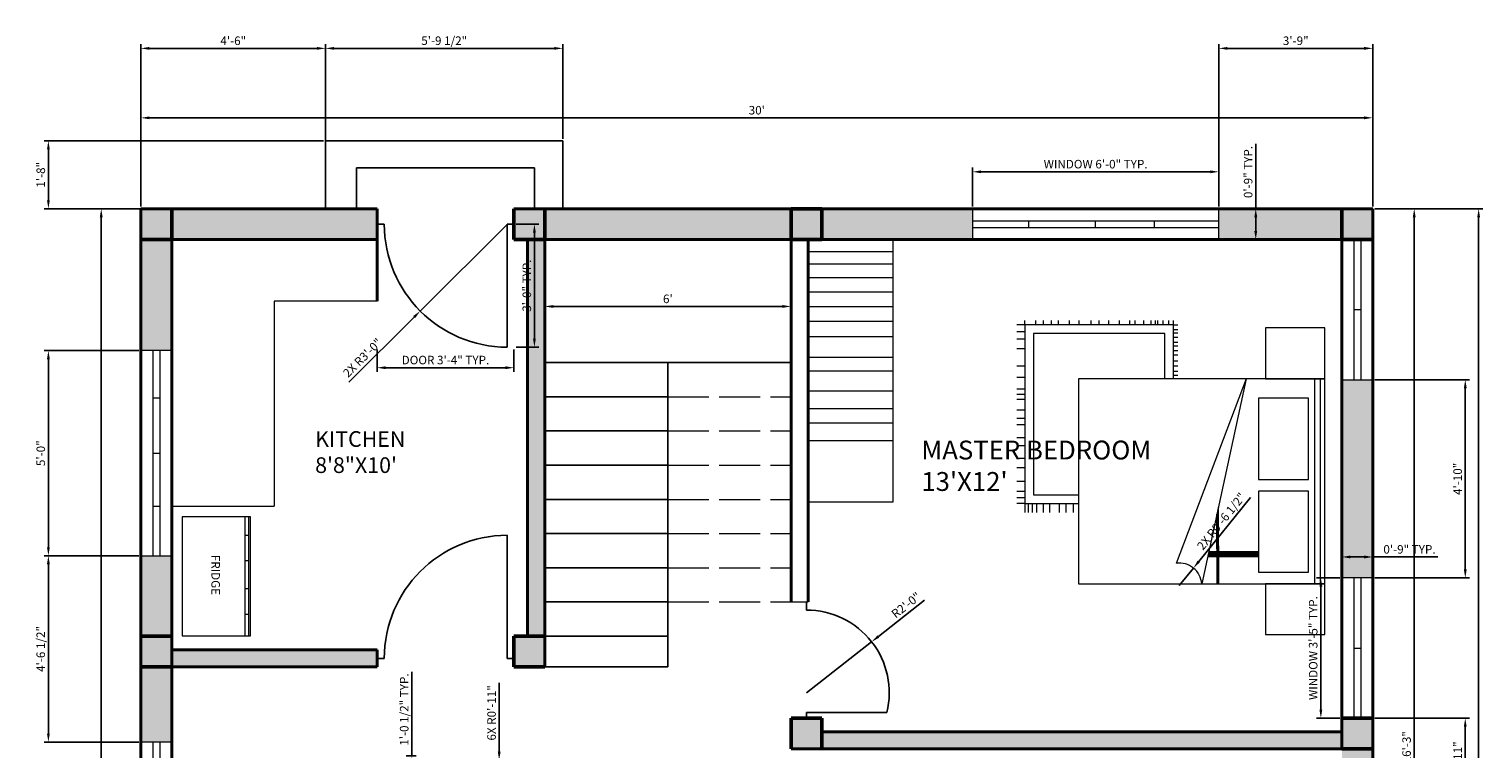
# Model space of a CAD drawing. Units: inches. Extents: x 599 to 1046, y 473 to 1020.
# Tile 2 of 2: x 621 to 1046, y 809 to 1020. Entities that reach past the tile are written whole.
import ezdxf

# ---------------------------------------------------------------- set-up
doc = ezdxf.new("R2010")
doc.units = ezdxf.units.IN
doc.linetypes.add('ACAD_ISO02W100', pattern=[15, 12, -3])
for name, color, linetype, lineweight in [('A-ANNO-DIMS', 2, 'Continuous', 18), ('A-ANNO-TEXT', 7, 'Continuous', 18), ('A-AREA-IDEN', 7, 'Continuous', 25), ('A-COLS', 7, 'Continuous', 50), ('A-COLS-PATT', 1, 'Continuous', 13), ('A-DOOR', 3, 'Continuous', 25), ('A-EQPM', 8, 'Continuous', 20), ('A-FLOR-CASE', 8, 'Continuous', 20), ('A-FLOR-STRS', 7, 'Continuous', 25), ('A-FLOR-STRS-OVHD', 7, 'ACAD_ISO02W100', 18), ('A-FURN', 8, 'Continuous', 18), ('A-GLAZ', 4, 'Continuous', 18), ('A-WALL', 7, 'Continuous', 40), ('A-WALL-PATT', 252, 'Continuous', 13)]:
    doc.layers.add(name, color=color, linetype=linetype, lineweight=lineweight)
doc.styles.get("Standard").update_dxf_attribs({"font": 'arial.ttf'})
doc.dimstyles.new('ISO-25', dxfattribs={"dimtxt": 2.5, "dimasz": 2.5, "dimexe": 1.25, "dimexo": 0.625, "dimtad": 1, "dimdec": 0, "dimlunit": 3, "dimtxsty": 'Standard', "dimcen": 2.5, "dimadec": 0, "dimazin": 0, "dimtfac": 1, "dimtdec": 0, "dimtmove": 0, "dimatfit": 3, "dimfxl": 1, "dimarcsym": 0})

# ---------------------------------------------------------------- blocks, each defined once
blk = doc.blocks.new('*D1')
at = {"layer": 'A-ANNO-DIMS', "color": 0, "lineweight": -2, "transparency": 16777216}
for p, q in [((771.31, 957.63), (771.31, 937.43)), ((843.31, 957.63), (843.31, 937.43)), ((773.81, 938.68), (840.81, 938.68))]:
    blk.add_line(p, q, dxfattribs=at)
at = {"layer": 'A-ANNO-DIMS', "color": 0, "transparency": 16777216}
for points in [[(773.81, 939.09), (773.81, 938.26), (771.31, 938.68)], [(840.81, 939.09), (840.81, 938.26), (843.31, 938.68)]]:
    blk.add_solid(points, dxfattribs=at)
at = {"layer": 'Defpoints', "color": 0, "transparency": 16777216}
for p in [(771.31, 958.26), (843.31, 958.26), (843.31, 938.68)]:
    blk.add_point(p, dxfattribs=at)
at = {"layer": 'A-ANNO-DIMS', "color": 0, "transparency": 16777216, "insert": (807.31, 940.58), "char_height": 2.5, "attachment_point": 5}
blk.add_mtext("6'", dxfattribs=at)
blk = doc.blocks.new('*D6')
at = {"layer": 'A-ANNO-DIMS', "color": 0, "lineweight": -2, "transparency": 16777216}
for p, q in [((1013.94, 967.26), (1026.69, 967.26)), ((1025.44, 654.76), (1025.44, 964.76)), ((1013.94, 652.26), (1026.69, 652.26))]:
    blk.add_line(p, q, dxfattribs=at)
at = {"layer": 'A-ANNO-DIMS', "color": 0, "transparency": 16777216}
for points in [[(1025.02, 964.76), (1025.86, 964.76), (1025.44, 967.26)], [(1025.02, 654.76), (1025.86, 654.76), (1025.44, 652.26)]]:
    blk.add_solid(points, dxfattribs=at)
at = {"layer": 'Defpoints', "color": 0, "transparency": 16777216}
for p in [(1013.31, 967.26), (1025.44, 967.26), (1013.31, 652.26)]:
    blk.add_point(p, dxfattribs=at)
at = {"layer": 'A-ANNO-DIMS', "color": 0, "transparency": 16777216, "insert": (1023.54, 809.76), "char_height": 2.5, "attachment_point": 5, "rotation": 90}
blk.add_mtext('26\'-3"', dxfattribs=at)
blk = doc.blocks.new('*D7')
at = {"layer": 'A-ANNO-DIMS', "color": 0, "lineweight": -2, "transparency": 16777216}
for p, q in [((1013.94, 967.26), (1045.52, 967.26)), ((1044.27, 964.76), (1044.27, 585.76)), ((1013.94, 583.26), (1045.52, 583.26))]:
    blk.add_line(p, q, dxfattribs=at)
at = {"layer": 'A-ANNO-DIMS', "color": 0, "transparency": 16777216}
for points in [[(1043.86, 964.76), (1044.69, 964.76), (1044.27, 967.26)], [(1043.86, 585.76), (1044.69, 585.76), (1044.27, 583.26)]]:
    blk.add_solid(points, dxfattribs=at)
at = {"layer": 'Defpoints', "color": 0, "transparency": 16777216}
for p in [(1013.31, 967.26), (1013.31, 583.26), (1044.27, 583.26)]:
    blk.add_point(p, dxfattribs=at)
at = {"layer": 'A-ANNO-DIMS', "color": 0, "transparency": 16777216, "insert": (1042.37, 775.26), "char_height": 2.5, "attachment_point": 5, "rotation": 90}
blk.add_mtext("32'", dxfattribs=at)
blk = doc.blocks.new('*D8')
at = {"layer": 'A-ANNO-DIMS', "color": 0, "lineweight": -2, "transparency": 16777216}
for p, q in [((652.69, 967.26), (640.46, 967.26)), ((641.71, 964.76), (641.71, 585.76)), ((652.69, 583.26), (640.46, 583.26))]:
    blk.add_line(p, q, dxfattribs=at)
at = {"layer": 'A-ANNO-DIMS', "color": 0, "transparency": 16777216}
for points in [[(641.29, 964.76), (642.13, 964.76), (641.71, 967.26)], [(641.29, 585.76), (642.13, 585.76), (641.71, 583.26)]]:
    blk.add_solid(points, dxfattribs=at)
at = {"layer": 'Defpoints', "color": 0, "transparency": 16777216}
for p in [(653.31, 967.26), (641.71, 583.26), (653.31, 583.26)]:
    blk.add_point(p, dxfattribs=at)
at = {"layer": 'A-ANNO-DIMS', "color": 0, "transparency": 16777216, "insert": (639.81, 775.26), "char_height": 2.5, "attachment_point": 5, "rotation": 90}
blk.add_mtext("32'", dxfattribs=at)
blk = doc.blocks.new('*D9')
at = {"layer": 'A-ANNO-DIMS', "color": 0, "lineweight": -2, "transparency": 16777216}
for p, q in [((653.31, 967.88), (653.31, 995.1)), ((1013.31, 967.88), (1013.31, 995.1)), ((655.81, 993.85), (1010.81, 993.85))]:
    blk.add_line(p, q, dxfattribs=at)
at = {"layer": 'A-ANNO-DIMS', "color": 0, "transparency": 16777216}
for points in [[(655.81, 994.27), (655.81, 993.43), (653.31, 993.85)], [(1010.81, 994.27), (1010.81, 993.43), (1013.31, 993.85)]]:
    blk.add_solid(points, dxfattribs=at)
at = {"layer": 'Defpoints', "color": 0, "transparency": 16777216}
for p in [(1013.31, 993.85), (653.31, 967.26), (1013.31, 967.26)]:
    blk.add_point(p, dxfattribs=at)
at = {"layer": 'A-ANNO-DIMS', "color": 0, "transparency": 16777216, "insert": (833.31, 995.75), "char_height": 2.5, "attachment_point": 5}
blk.add_mtext("30'", dxfattribs=at)
blk = doc.blocks.new('BED-DOUBLE-ENSEMBLE')
for p, q in [((0, 77.06), (0, 17.06)), ((72, 77.06), (0, 77.06)), ((1.3, 77.06), (1.3, 17.06)), ((2.94, 77.06), (2.94, 17.06)), ((22.99, 17.06), (36, 77.06)), ((30.98, 77.06), (31.13, 54.62)), ((31.25, 55.16), (31.25, 77.06)), ((31.34, 55.57), (31.34, 77.06)), ((31.5, 77.06), (31.57, 56.64)), ((72, 17.06), (72, 77.06)), ((19.36, 69.18), (34.29, 69.19)), ((19.36, 68.78), (34.21, 68.79)), ((19.36, 68.38), (34.12, 68.39)), ((19.36, 68.04), (34.05, 68.05)), ((22.99, 17.06), (43.43, 71.06)), ((19.36, 67.69), (33.97, 67.7)), ((73.56, 53.54), (73.56, 56.2)), ((75.7, 53.54), (75.7, 56.2)), ((77.64, 53.54), (77.64, 56.2)), ((80.52, 53.54), (80.52, 56.2)), ((82.37, 53.54), (82.37, 56.2)), ((84.31, 53.54), (84.31, 56.2)), ((85.54, 53.54), (85.54, 56.2)), ((86.7, 53.54), (86.7, 56.2)), ((87.67, 53.54), (87.67, 56.2)), ((87.67, 53.54), (72, 53.54)), ((85.18, 51.05), (72, 51.05)), ((85.18, 3.81), (85.18, 51.05)), ((87.67, 1.32), (87.67, 53.54)), ((87.67, 53.54), (90.06, 53.54)), ((87.67, 51.93), (90.06, 51.93)), ((87.67, 50.03), (90.06, 50.03)), ((87.67, 47.15), (90.06, 47.15)), ((87.67, 43.16), (90.06, 43.16)), ((87.67, 40.35), (90.06, 40.35)), ((87.67, 36.69), (90.06, 36.69)), ((87.67, 34.33), (90.06, 34.33)), ((87.67, 30.54), (90.06, 30.54)), ((87.67, 28.71), (90.06, 28.71)), ((87.67, 26.29), (90.06, 26.29)), ((87.67, 23.15), (90.06, 23.15)), ((87.67, 21.64), (90.06, 21.64)), ((0, 17.06), (72, 17.06)), ((44.26, 17.06), (44.26, 1.32)), ((46.75, 17.06), (46.75, 3.81)), ((87.67, 20.07), (90.06, 20.07)), ((44.26, 16), (42.95, 16)), ((44.26, 14.88), (42.95, 14.88)), ((44.26, 13.3), (42.95, 13.3)), ((87.67, 16.74), (90.06, 16.74)), ((87.67, 13.4), (90.06, 13.4)), ((44.26, 11.8), (42.95, 11.8)), ((44.26, 10.06), (42.95, 10.06)), ((44.26, 8.76), (42.95, 8.76)), ((44.26, 7.43), (42.95, 7.43)), ((44.26, 6.36), (42.95, 6.36)), ((44.26, 4.95), (42.95, 4.95)), ((87.67, 8.34), (90.06, 8.34)), ((87.67, 5.52), (90.06, 5.52)), ((44.26, 3.6), (42.95, 3.6)), ((44.26, 2.68), (42.95, 2.68)), ((44.26, 1.32), (42.95, 1.32)), ((44.26, 1.32), (87.67, 1.32)), ((44.26, 1.32), (44.26, 0)), ((45.56, 1.32), (45.56, 0)), ((46.75, 3.81), (85.18, 3.81)), ((47.24, 1.32), (47.24, 0)), ((48.78, 1.32), (48.78, 0)), ((49.52, 1.32), (49.52, 0)), ((50.72, 1.32), (50.72, 0)), ((52.92, 1.32), (52.92, 0)), ((55.47, 1.32), (55.47, 0)), ((56.97, 1.32), (56.97, 0)), ((60.04, 1.32), (60.04, 0)), ((63.18, 1.32), (63.18, 0)), ((65.96, 1.32), (65.96, 0)), ((68.28, 1.32), (68.28, 0)), ((71.81, 1.32), (71.81, 0)), ((74.68, 1.32), (74.68, 0)), ((77.82, 1.32), (77.82, 0)), ((79.85, 1.32), (79.85, 0)), ((82.2, 1.32), (82.2, 0)), ((84.49, 1.32), (84.49, 0)), ((87.67, 3.36), (90.06, 3.36)), ((87.67, 1.32), (87.67, 0)), ((87.67, 1.32), (87.67, 0)), ((87.67, 1.32), (90.06, 1.32))]:
    blk.add_line(p, q)
for points in [[(0, 77.06), (17.35, 77.06), (17.35, 91.9), (0, 91.9)], [(4.8, 49.9), (19.36, 49.9), (19.36, 73.67), (4.8, 73.67)], [(4.8, 22.77), (19.36, 22.77), (19.36, 46.55), (4.8, 46.55)], [(0, 2.22), (17.35, 2.22), (17.35, 17.06), (0, 17.06)]]:
    blk.add_lwpolyline(points, close=True)
blk.add_arc((42.53, 77.54), 6.55, 184.2463, 277.8518)
blk = doc.blocks.new('WARDROBE-BEDROOM')
for p, q in [((0, 73.38), (24.73, 73.38)), ((0, 69.72), (24.73, 69.72)), ((0, 65.72), (24.73, 65.72)), ((0, 61.6), (24.73, 61.6)), ((0, 57.26), (24.73, 57.26)), ((0, 52.97), (24.73, 52.97)), ((0, 48.49), (24.73, 48.49)), ((0, 42.41), (24.73, 42.41)), ((0, 38.43), (24.73, 38.43)), ((0, 32.59), (24.73, 32.59)), ((0, 27.44), (24.73, 27.44)), ((0, 23.23), (24.73, 23.23)), ((0, 18.05), (24.73, 18.05))]:
    blk.add_line(p, q)
blk.add_lwpolyline([(0, 76.86), (24.73, 76.86), (24.73, 0), (0, 0)], close=True)
blk = doc.blocks.new('WIN-72IN')
for p, q in [((3.5, 72), (3.5, 0)), ((5.5, 72), (5.5, 0)), ((3.5, 55.48), (5.5, 55.48)), ((3.5, 36), (5.5, 36)), ((3.5, 18.8), (5.5, 18.8))]:
    blk.add_line(p, q)
blk.add_lwpolyline([(0, 72), (0, 0), (9, 0), (9, 72)], close=True)
blk = doc.blocks.new('WIN-41IN')
for p, q in [((3.5, 41), (3.5, 0)), ((5.5, 41), (5.5, 0)), ((3.5, 20.5), (5.5, 20.5))]:
    blk.add_line(p, q)
blk.add_lwpolyline([(0, 41), (0, 0), (9, 0), (9, 41)], close=True)
blk = doc.blocks.new('DOOR-SINGLE-36IN')
for p, q in [((0, 36), (2.13, 36)), ((38, 36), (38, 0)), ((38, 36), (40, 36))]:
    blk.add_line(p, q)
blk.add_arc((38.13, 36), 36, 180, 269.8005)
blk = doc.blocks.new('*D18')
at = {"layer": 'A-ANNO-DIMS', "color": 0, "lineweight": -2, "transparency": 16777216}
for p, q in [((732.5, 807.24), (732.5, 831.82)), ((730.82, 807.24), (733.75, 807.24)), ((732.5, 797.39), (732.5, 804.74)), ((730.82, 794.89), (733.75, 794.89))]:
    blk.add_line(p, q, dxfattribs=at)
at = {"layer": 'A-ANNO-DIMS', "color": 0, "transparency": 16777216}
for points in [[(732.08, 804.74), (732.91, 804.74), (732.5, 807.24)], [(732.08, 797.39), (732.91, 797.39), (732.5, 794.89)]]:
    blk.add_solid(points, dxfattribs=at)
at = {"layer": 'Defpoints', "color": 0, "transparency": 16777216}
for p in [(730.19, 807.24), (732.5, 807.24), (730.19, 794.89)]:
    blk.add_point(p, dxfattribs=at)
at = {"layer": 'A-ANNO-DIMS', "color": 0, "transparency": 16777216, "insert": (730.58, 820.78), "char_height": 2.5, "attachment_point": 5, "rotation": 90}
blk.add_mtext('1\'-0 1/2" TYP.', dxfattribs=at)
blk = doc.blocks.new('*D19')
at = {"layer": 'A-ANNO-DIMS', "color": 0, "lineweight": -2, "transparency": 16777216}
for p, q in [((896.33, 967.88), (896.33, 979.31)), ((965.83, 978.06), (898.83, 978.06)), ((968.33, 967.88), (968.33, 979.31))]:
    blk.add_line(p, q, dxfattribs=at)
at = {"layer": 'A-ANNO-DIMS', "color": 0, "transparency": 16777216}
for points in [[(898.83, 978.48), (898.83, 977.64), (896.33, 978.06)], [(965.83, 978.48), (965.83, 977.64), (968.33, 978.06)]]:
    blk.add_solid(points, dxfattribs=at)
at = {"layer": 'Defpoints', "color": 0, "transparency": 16777216}
for p in [(896.33, 978.06), (896.33, 967.26), (968.33, 967.26)]:
    blk.add_point(p, dxfattribs=at)
at = {"layer": 'A-ANNO-DIMS', "color": 0, "transparency": 16777216, "insert": (932.33, 979.98), "char_height": 2.5, "attachment_point": 5}
blk.add_mtext('WINDOW 6\'-0" TYP.', dxfattribs=at)
blk = doc.blocks.new('*D20')
at = {"layer": 'A-ANNO-DIMS', "color": 0, "lineweight": -2, "transparency": 16777216}
for p, q in [((979.13, 967.26), (979.13, 986.25)), ((968.96, 967.26), (980.38, 967.26)), ((979.13, 960.76), (979.13, 964.76)), ((968.96, 958.26), (980.38, 958.26))]:
    blk.add_line(p, q, dxfattribs=at)
at = {"layer": 'A-ANNO-DIMS', "color": 0, "transparency": 16777216}
for points in [[(978.72, 964.76), (979.55, 964.76), (979.13, 967.26)], [(978.72, 960.76), (979.55, 960.76), (979.13, 958.26)]]:
    blk.add_solid(points, dxfattribs=at)
at = {"layer": 'Defpoints', "color": 0, "transparency": 16777216}
for p in [(968.33, 967.26), (979.13, 967.26), (968.33, 958.26)]:
    blk.add_point(p, dxfattribs=at)
at = {"layer": 'A-ANNO-DIMS', "color": 0, "transparency": 16777216, "insert": (977.23, 978), "char_height": 2.5, "attachment_point": 5, "rotation": 90}
blk.add_mtext('0\'-9" TYP.', dxfattribs=at)
blk = doc.blocks.new('*D21')
at = {"layer": 'A-ANNO-DIMS', "color": 0, "lineweight": -2, "transparency": 16777216}
for p, q in [((722.31, 926.13), (722.31, 919.51)), ((762.31, 926.13), (762.31, 919.51)), ((724.81, 920.76), (759.81, 920.76))]:
    blk.add_line(p, q, dxfattribs=at)
at = {"layer": 'A-ANNO-DIMS', "color": 0, "transparency": 16777216}
for points in [[(724.81, 921.18), (724.81, 920.34), (722.31, 920.76)], [(759.81, 921.18), (759.81, 920.34), (762.31, 920.76)]]:
    blk.add_solid(points, dxfattribs=at)
at = {"layer": 'Defpoints', "color": 0, "transparency": 16777216}
for p in [(722.31, 926.76), (762.31, 926.76), (762.31, 920.76)]:
    blk.add_point(p, dxfattribs=at)
at = {"layer": 'A-ANNO-DIMS', "color": 0, "transparency": 16777216, "insert": (742.31, 922.68), "char_height": 2.5, "attachment_point": 5}
blk.add_mtext('DOOR 3\'-4" TYP.', dxfattribs=at)
blk = doc.blocks.new('*D22')
at = {"layer": 'A-ANNO-DIMS', "color": 0, "lineweight": -2, "transparency": 16777216}
for p, q in [((762.94, 962.76), (769.56, 962.76)), ((768.31, 929.26), (768.31, 960.26)), ((762.94, 926.76), (769.56, 926.76))]:
    blk.add_line(p, q, dxfattribs=at)
at = {"layer": 'A-ANNO-DIMS', "color": 0, "transparency": 16777216}
for points in [[(767.9, 960.26), (768.73, 960.26), (768.31, 962.76)], [(767.9, 929.26), (768.73, 929.26), (768.31, 926.76)]]:
    blk.add_solid(points, dxfattribs=at)
at = {"layer": 'Defpoints', "color": 0, "transparency": 16777216}
for p in [(762.31, 962.76), (768.31, 962.76), (762.31, 926.76)]:
    blk.add_point(p, dxfattribs=at)
at = {"layer": 'A-ANNO-DIMS', "color": 0, "transparency": 16777216, "insert": (766.41, 944.76), "char_height": 2.5, "attachment_point": 5, "rotation": 90}
blk.add_mtext('3\'-0" TYP.', dxfattribs=at)
blk = doc.blocks.new('*D27')
at = {"layer": 'A-ANNO-DIMS', "color": 0, "lineweight": -2, "transparency": 16777216}
for p, q in [((1003.69, 859.26), (996.91, 859.26)), ((998.16, 820.76), (998.16, 856.76)), ((1003.69, 818.26), (996.91, 818.26))]:
    blk.add_line(p, q, dxfattribs=at)
at = {"layer": 'A-ANNO-DIMS', "color": 0, "transparency": 16777216}
for points in [[(997.75, 856.76), (998.58, 856.76), (998.16, 859.26)], [(997.75, 820.76), (998.58, 820.76), (998.16, 818.26)]]:
    blk.add_solid(points, dxfattribs=at)
at = {"layer": 'Defpoints', "color": 0, "transparency": 16777216}
for p in [(998.16, 859.26), (1004.31, 859.26), (1004.31, 818.26)]:
    blk.add_point(p, dxfattribs=at)
at = {"layer": 'A-ANNO-DIMS', "color": 0, "transparency": 16777216, "insert": (996.24, 838.76), "char_height": 2.5, "attachment_point": 5, "rotation": 90}
blk.add_mtext('WINDOW 3\'-5" TYP.', dxfattribs=at)
blk = doc.blocks.new('*D28')
at = {"layer": 'A-ANNO-DIMS', "color": 0, "lineweight": -2, "transparency": 16777216}
for p, q in [((1004.31, 859.88), (1004.31, 866.66)), ((1006.81, 865.41), (1010.81, 865.41)), ((1013.31, 859.88), (1013.31, 866.66)), ((1013.31, 865.41), (1032.3, 865.41))]:
    blk.add_line(p, q, dxfattribs=at)
at = {"layer": 'A-ANNO-DIMS', "color": 0, "transparency": 16777216}
for points in [[(1006.81, 865.83), (1006.81, 864.99), (1004.31, 865.41)], [(1010.81, 865.83), (1010.81, 864.99), (1013.31, 865.41)]]:
    blk.add_solid(points, dxfattribs=at)
at = {"layer": 'Defpoints', "color": 0, "transparency": 16777216}
for p in [(1013.31, 865.41), (1004.31, 859.26), (1013.31, 859.26)]:
    blk.add_point(p, dxfattribs=at)
at = {"layer": 'A-ANNO-DIMS', "color": 0, "transparency": 16777216, "insert": (1024.06, 867.31), "char_height": 2.5, "attachment_point": 5}
blk.add_mtext('0\'-9" TYP.', dxfattribs=at)
blk = doc.blocks.new('*D31')
at = {"layer": 'A-ANNO-DIMS', "color": 0, "lineweight": -2, "transparency": 16777216}
for p, q in [((707.27, 987.74), (707.27, 1015.42)), ((709.77, 1014.17), (774.13, 1014.17)), ((776.63, 987.74), (776.63, 1015.42))]:
    blk.add_line(p, q, dxfattribs=at)
at = {"layer": 'A-ANNO-DIMS', "color": 0, "transparency": 16777216}
for points in [[(709.77, 1014.59), (709.77, 1013.75), (707.27, 1014.17)], [(774.13, 1014.59), (774.13, 1013.75), (776.63, 1014.17)]]:
    blk.add_solid(points, dxfattribs=at)
at = {"layer": 'Defpoints', "color": 0, "transparency": 16777216}
for p in [(776.63, 1014.17), (707.27, 987.12), (776.63, 987.12)]:
    blk.add_point(p, dxfattribs=at)
at = {"layer": 'A-ANNO-DIMS', "color": 0, "transparency": 16777216, "insert": (741.95, 1016.09), "char_height": 2.5, "attachment_point": 5}
blk.add_mtext('5\'-9 1/2"', dxfattribs=at)
blk = doc.blocks.new('*D32')
at = {"layer": 'A-ANNO-DIMS', "color": 0, "lineweight": -2, "transparency": 16777216}
for p, q in [((706.65, 987.12), (625.01, 987.12)), ((626.26, 969.76), (626.26, 984.62)), ((706.65, 967.26), (625.01, 967.26))]:
    blk.add_line(p, q, dxfattribs=at)
at = {"layer": 'A-ANNO-DIMS', "color": 0, "transparency": 16777216}
for points in [[(625.85, 984.62), (626.68, 984.62), (626.26, 987.12)], [(625.85, 969.76), (626.68, 969.76), (626.26, 967.26)]]:
    blk.add_solid(points, dxfattribs=at)
at = {"layer": 'Defpoints', "color": 0, "transparency": 16777216}
for p in [(626.26, 987.12), (707.27, 987.12), (707.27, 967.26)]:
    blk.add_point(p, dxfattribs=at)
at = {"layer": 'A-ANNO-DIMS', "color": 0, "transparency": 16777216, "insert": (624.36, 977.19), "char_height": 2.5, "attachment_point": 5, "rotation": 90}
blk.add_mtext('1\'-8"', dxfattribs=at)
blk = doc.blocks.new('*D33')
at = {"layer": 'A-ANNO-DIMS', "color": 0, "lineweight": -2, "transparency": 16777216}
for p, q in [((653.31, 967.88), (653.31, 1015.42)), ((655.81, 1014.17), (704.77, 1014.17)), ((707.27, 967.88), (707.27, 1015.42))]:
    blk.add_line(p, q, dxfattribs=at)
at = {"layer": 'A-ANNO-DIMS', "color": 0, "transparency": 16777216}
for points in [[(655.81, 1014.59), (655.81, 1013.75), (653.31, 1014.17)], [(704.77, 1014.59), (704.77, 1013.75), (707.27, 1014.17)]]:
    blk.add_solid(points, dxfattribs=at)
at = {"layer": 'Defpoints', "color": 0, "transparency": 16777216}
for p in [(707.27, 1014.17), (653.31, 967.26), (707.27, 967.26)]:
    blk.add_point(p, dxfattribs=at)
at = {"layer": 'A-ANNO-DIMS', "color": 0, "transparency": 16777216, "insert": (680.29, 1016.07), "char_height": 2.5, "attachment_point": 5}
blk.add_mtext('4\'-6"', dxfattribs=at)
blk = doc.blocks.new('*D34')
at = {"layer": 'A-ANNO-DIMS', "color": 0, "lineweight": -2, "transparency": 16777216}
for p, q in [((652.69, 925.76), (625.01, 925.76)), ((626.26, 923.26), (626.26, 868.26)), ((652.69, 865.76), (625.01, 865.76))]:
    blk.add_line(p, q, dxfattribs=at)
at = {"layer": 'A-ANNO-DIMS', "color": 0, "transparency": 16777216}
for points in [[(625.85, 923.26), (626.68, 923.26), (626.26, 925.76)], [(625.85, 868.26), (626.68, 868.26), (626.26, 865.76)]]:
    blk.add_solid(points, dxfattribs=at)
at = {"layer": 'Defpoints', "color": 0, "transparency": 16777216}
for p in [(653.31, 925.76), (626.26, 865.76), (653.31, 865.76)]:
    blk.add_point(p, dxfattribs=at)
at = {"layer": 'A-ANNO-DIMS', "color": 0, "transparency": 16777216, "insert": (624.36, 895.76), "char_height": 2.5, "attachment_point": 5, "rotation": 90}
blk.add_mtext('5\'-0"', dxfattribs=at)
blk = doc.blocks.new('*D38')
at = {"layer": 'A-ANNO-DIMS', "color": 0, "lineweight": -2, "transparency": 16777216}
for p, q in [((652.69, 865.76), (625.01, 865.76)), ((626.26, 863.26), (626.26, 813.76)), ((652.69, 811.26), (625.01, 811.26))]:
    blk.add_line(p, q, dxfattribs=at)
at = {"layer": 'A-ANNO-DIMS', "color": 0, "transparency": 16777216}
for points in [[(625.85, 863.26), (626.68, 863.26), (626.26, 865.76)], [(625.85, 813.76), (626.68, 813.76), (626.26, 811.26)]]:
    blk.add_solid(points, dxfattribs=at)
at = {"layer": 'Defpoints', "color": 0, "transparency": 16777216}
for p in [(653.31, 865.76), (626.26, 811.26), (653.31, 811.26)]:
    blk.add_point(p, dxfattribs=at)
at = {"layer": 'A-ANNO-DIMS', "color": 0, "transparency": 16777216, "insert": (624.35, 838.51), "char_height": 2.5, "attachment_point": 5, "rotation": 90}
blk.add_mtext('4\'-6 1/2"', dxfattribs=at)
blk = doc.blocks.new('*D40')
at = {"layer": 'A-ANNO-DIMS', "color": 0, "lineweight": -2, "transparency": 16777216}
for p, q in [((968.33, 967.88), (968.33, 1015.42)), ((970.83, 1014.17), (1010.81, 1014.17)), ((1013.31, 967.88), (1013.31, 1015.42))]:
    blk.add_line(p, q, dxfattribs=at)
at = {"layer": 'A-ANNO-DIMS', "color": 0, "transparency": 16777216}
for points in [[(970.83, 1014.59), (970.83, 1013.75), (968.33, 1014.17)], [(1010.81, 1014.59), (1010.81, 1013.75), (1013.31, 1014.17)]]:
    blk.add_solid(points, dxfattribs=at)
at = {"layer": 'Defpoints', "color": 0, "transparency": 16777216}
for p in [(1013.31, 1014.17), (968.33, 967.26), (1013.31, 967.26)]:
    blk.add_point(p, dxfattribs=at)
at = {"layer": 'A-ANNO-DIMS', "color": 0, "transparency": 16777216, "insert": (990.82, 1016.07), "char_height": 2.5, "attachment_point": 5}
blk.add_mtext('3\'-9"', dxfattribs=at)
blk = doc.blocks.new('*D41')
at = {"layer": 'A-ANNO-DIMS', "color": 0, "lineweight": -2, "transparency": 16777216}
for p, q in [((1013.94, 917.26), (1041.61, 917.26)), ((1040.36, 914.76), (1040.36, 861.76)), ((1013.94, 859.26), (1041.61, 859.26))]:
    blk.add_line(p, q, dxfattribs=at)
at = {"layer": 'A-ANNO-DIMS', "color": 0, "transparency": 16777216}
for points in [[(1039.95, 914.76), (1040.78, 914.76), (1040.36, 917.26)], [(1039.95, 861.76), (1040.78, 861.76), (1040.36, 859.26)]]:
    blk.add_solid(points, dxfattribs=at)
at = {"layer": 'Defpoints', "color": 0, "transparency": 16777216}
for p in [(1013.31, 917.26), (1013.31, 859.26), (1040.36, 859.26)]:
    blk.add_point(p, dxfattribs=at)
at = {"layer": 'A-ANNO-DIMS', "color": 0, "transparency": 16777216, "insert": (1038.46, 888.26), "char_height": 2.5, "attachment_point": 5, "rotation": 90}
blk.add_mtext('4\'-10"', dxfattribs=at)
blk = doc.blocks.new('*D42')
at = {"layer": 'A-ANNO-DIMS', "color": 0, "lineweight": -2, "transparency": 16777216}
for p, q in [((1013.94, 818.26), (1041.61, 818.26)), ((1040.36, 815.76), (1040.36, 797.76)), ((1013.94, 795.26), (1041.61, 795.26))]:
    blk.add_line(p, q, dxfattribs=at)
at = {"layer": 'A-ANNO-DIMS', "color": 0, "transparency": 16777216}
for points in [[(1039.95, 815.76), (1040.78, 815.76), (1040.36, 818.26)], [(1039.95, 797.76), (1040.78, 797.76), (1040.36, 795.26)]]:
    blk.add_solid(points, dxfattribs=at)
at = {"layer": 'Defpoints', "color": 0, "transparency": 16777216}
for p in [(1013.31, 818.26), (1013.31, 795.26), (1040.36, 795.26)]:
    blk.add_point(p, dxfattribs=at)
at = {"layer": 'A-ANNO-DIMS', "color": 0, "transparency": 16777216, "insert": (1038.48, 806.76), "char_height": 2.5, "attachment_point": 5, "rotation": 90}
blk.add_mtext('1\'-11"', dxfattribs=at)
blk = doc.blocks.new('*D44')
at = {"layer": 'A-ANNO-DIMS', "color": 0, "lineweight": -2, "transparency": 16777216}
for p, q in [((882.35, 852.75), (868.84, 842.14)), ((847.81, 825.65), (866.87, 840.6))]:
    blk.add_line(p, q, dxfattribs=at)
at = {"layer": 'A-ANNO-DIMS', "color": 0, "transparency": 16777216}
blk.add_solid([(868.58, 842.47), (869.1, 841.81), (866.87, 840.6)], dxfattribs=at)
at = {"layer": 'Defpoints', "color": 0, "transparency": 16777216}
for p in [(866.87, 840.6), (847.81, 825.65)]:
    blk.add_point(p, dxfattribs=at)
at = {"layer": 'A-ANNO-DIMS', "color": 0, "transparency": 16777216, "insert": (877.13, 851.07), "char_height": 2.5, "attachment_point": 5, "rotation": 38.1173}
blk.add_mtext('R2\'-0"', dxfattribs=at)
blk = doc.blocks.new('*D46')
at = {"layer": 'A-ANNO-DIMS', "color": 0, "lineweight": -2, "transparency": 16777216}
for p, q in [((760.44, 962.76), (734.94, 937.35)), ((714.08, 916.56), (733.17, 935.58))]:
    blk.add_line(p, q, dxfattribs=at)
at = {"layer": 'A-ANNO-DIMS', "color": 0, "transparency": 16777216}
blk.add_solid([(732.87, 935.88), (733.46, 935.29), (734.94, 937.35)], dxfattribs=at)
at = {"layer": 'Defpoints', "color": 0, "transparency": 16777216}
for p in [(760.44, 962.76), (734.94, 937.35)]:
    blk.add_point(p, dxfattribs=at)
at = {"layer": 'A-ANNO-DIMS', "color": 0, "transparency": 16777216, "insert": (718.3, 923.45), "char_height": 2.5, "attachment_point": 5, "rotation": 44.8993}
blk.add_mtext('2X R3\'-0"', dxfattribs=at)
blk = doc.blocks.new('*D47')
at = {"layer": 'A-ANNO-DIMS', "color": 0, "lineweight": -2, "transparency": 16777216}
for p, q in [((758.01, 828.61), (758.01, 808.5)), ((758.01, 794.78), (758.01, 806))]:
    blk.add_line(p, q, dxfattribs=at)
at = {"layer": 'A-ANNO-DIMS', "color": 0, "transparency": 16777216}
blk.add_solid([(757.59, 808.5), (758.43, 808.5), (758.01, 806)], dxfattribs=at)
at = {"layer": 'Defpoints', "color": 0, "transparency": 16777216}
for p in [(758.01, 806), (758.01, 794.78)]:
    blk.add_point(p, dxfattribs=at)
at = {"layer": 'A-ANNO-DIMS', "color": 0, "transparency": 16777216, "insert": (756.11, 819.81), "char_height": 2.5, "attachment_point": 5, "rotation": 89.9975}
blk.add_mtext('6X R0\'-11"', dxfattribs=at)
blk = doc.blocks.new('*D48')
at = {"layer": 'A-ANNO-DIMS', "color": 0, "lineweight": -2, "transparency": 16777216}
for p, q in [((977.59, 882.78), (962.48, 864.09)), ((956.79, 857.06), (960.91, 862.15))]:
    blk.add_line(p, q, dxfattribs=at)
at = {"layer": 'A-ANNO-DIMS', "color": 0, "transparency": 16777216}
blk.add_solid([(962.16, 864.36), (962.81, 863.83), (960.91, 862.15)], dxfattribs=at)
at = {"layer": 'Defpoints', "color": 0, "transparency": 16777216}
for p in [(960.91, 862.15), (956.79, 857.06)]:
    blk.add_point(p, dxfattribs=at)
at = {"layer": 'A-ANNO-DIMS', "color": 0, "transparency": 16777216, "insert": (969.33, 875.62), "char_height": 2.5, "attachment_point": 5, "rotation": 51.0506}
blk.add_mtext('2X R0\'-6 1/2"', dxfattribs=at)

msp = doc.modelspace()

# ---------------------------------------------------------------- hatches: boundary and pattern name
at = {"layer": 'A-COLS-PATT'}
h = msp.add_hatch(color=256, dxfattribs=at)
h.dxf.hatch_style = 1
h.paths.add_polyline_path([(662.31, 967.26), (653.31, 967.26), (653.31, 958.26), (662.31, 958.26)])
h.paths.add_polyline_path([(852.31, 967.26), (843.31, 967.26), (843.31, 958.26), (852.31, 958.26)])
h.paths.add_polyline_path([(771.31, 842.26), (762.31, 842.26), (762.31, 833.26), (771.31, 833.26)])
h.paths.add_polyline_path([(771.31, 967.26), (762.31, 967.26), (762.31, 958.26), (771.31, 958.26)])
h.paths.add_polyline_path([(662.31, 842.26), (653.31, 842.26), (653.31, 833.26), (662.31, 833.26)])
h.paths.add_polyline_path([(852.31, 818.26), (843.31, 818.26), (843.31, 809.26), (852.31, 809.26)])
h.paths.add_polyline_path([(1013.31, 967.26), (1004.31, 967.26), (1004.31, 958.26), (1013.31, 958.26)])
h.paths.add_polyline_path([(662.31, 592.26), (653.31, 592.26), (653.31, 583.26), (662.31, 583.26)])
h = msp.add_hatch(color=256, dxfattribs=at)
h.dxf.hatch_style = 1
h.paths.add_polyline_path([(662.31, 717.26), (653.31, 717.26), (653.31, 708.26), (662.31, 708.26)])
h.paths.add_polyline_path([(872.31, 717.26), (862.31, 717.26), (862.31, 708.26), (872.31, 708.26)])
h.paths.add_polyline_path([(872.31, 592.26), (862.31, 592.26), (862.31, 583.26), (872.31, 583.26)])
h.paths.add_polyline_path([(1013.31, 661.26), (1004.31, 661.26), (1004.31, 652.26), (1013.31, 652.26)])
h.paths.add_polyline_path([(1013.31, 818.26), (1004.31, 818.26), (1004.31, 809.26), (1013.31, 809.26)])
at = {"layer": 'A-WALL-PATT'}
h = msp.add_hatch(color=256, dxfattribs=at)
h.dxf.hatch_style = 1
h.paths.add_polyline_path([(662.31, 865.76), (653.31, 865.76), (653.31, 842.26), (662.31, 842.26)])
h.paths.add_polyline_path([(662.31, 833.26), (653.31, 833.26), (653.31, 811.26), (662.31, 811.26)])
h.paths.add_polyline_path([(722.31, 838.26), (662.31, 838.26), (662.31, 833.26), (722.31, 833.26)])
h.paths.add_polyline_path([(662.31, 739.26), (653.31, 739.26), (653.31, 717.26), (662.31, 717.26)])
h.paths.add_polyline_path([(662.31, 708.26), (653.31, 708.26), (653.31, 651.68), (662.31, 651.68), (662.31, 676.26), (692.31, 676.26), (692.31, 681.26), (662.31, 681.26)])
h.paths.add_polyline_path([(662.31, 627.68), (653.31, 627.68), (653.31, 592.26), (662.31, 592.26)])
h.paths.add_polyline_path([(766.2, 592.26), (730.31, 592.26), (730.31, 712.26), (822.31, 712.26), (822.31, 717.26), (724.31, 717.26), (724.31, 676.26), (724.31, 592.26), (662.31, 592.26), (662.31, 583.26), (766.2, 583.26)])
h.paths.add_polyline_path([(872.31, 708.26), (862.31, 708.26), (862.31, 592.26), (872.31, 592.26)])
h.paths.add_polyline_path([(1013.31, 809.26), (1004.31, 809.26), (1004.31, 795.26), (1013.31, 795.26)])
h.paths.add_polyline_path([(1004.31, 814.26), (852.31, 814.26), (852.31, 809.26), (1004.31, 809.26)])
h.paths.add_polyline_path([(843.31, 967.26), (771.31, 967.26), (771.31, 958.26), (843.31, 958.26)])
h.paths.add_polyline_path([(771.31, 958.26), (766.31, 958.26), (766.31, 842.26), (771.31, 842.26)])
h.paths.add_polyline_path([(722.31, 967.26), (662.31, 967.26), (662.31, 958.26), (722.31, 958.26)])
h.paths.add_polyline_path([(662.31, 958.26), (653.31, 958.26), (653.31, 925.76), (662.31, 925.76)])
h.paths.add_polyline_path([(896.33, 967.26), (852.31, 967.26), (852.31, 958.26), (873.04, 958.26), (896.33, 958.26)])
h.paths.add_polyline_path([(1004.31, 967.26), (968.33, 967.26), (968.33, 958.26), (1004.31, 958.26)])
h.paths.add_polyline_path([(1013.31, 917.26), (1004.31, 917.26), (1004.31, 859.26), (1013.31, 859.26)])
h.paths.add_polyline_path([(1013.31, 723.26), (1004.31, 723.26), (1004.31, 709.26), (1000.32, 709.26), (1000.32, 700.26), (1013.31, 700.26)])
h.paths.add_polyline_path([(872.31, 749.26), (862.31, 749.26), (862.31, 717.26), (872.31, 717.26)])
h.paths.add_polyline_path([(862.31, 592.26), (838.2, 592.26), (838.2, 583.26), (862.31, 583.26)])
h.paths.add_polyline_path([(928.32, 709.26), (924.31, 709.26), (924.31, 700.26), (928.32, 700.26)])

# ---------------------------------------------------------------- linework, layer by layer
at = {"layer": 'A-COLS'}
for p, q in [((662.31, 958.26), (662.31, 967.26)), ((762.31, 967.26), (762.31, 958.26)), ((771.31, 958.26), (771.31, 967.26)), ((852.31, 967.26), (843.31, 967.26)), ((843.31, 967.26), (843.31, 958.26)), ((852.31, 958.26), (852.31, 967.26)), ((1004.31, 967.26), (1004.31, 958.26)), ((653.31, 958.26), (662.31, 958.26)), ((762.31, 958.26), (771.31, 958.26)), ((843.31, 958.26), (852.31, 958.26)), ((1004.31, 958.26), (1013.31, 958.26)), ((662.31, 842.26), (653.31, 842.26)), ((771.31, 842.26), (762.31, 842.26)), ((762.31, 842.26), (762.31, 833.26)), ((653.31, 833.26), (662.31, 833.26)), ((762.31, 833.26), (771.31, 833.26)), ((771.31, 833.26), (766.31, 833.26)), ((843.31, 809.26), (843.31, 818.26)), ((852.31, 818.26), (843.31, 818.26)), ((852.31, 809.26), (852.31, 818.26)), ((1013.31, 818.26), (1004.31, 818.26)), ((1004.31, 809.26), (1013.31, 809.26))]:
    msp.add_line(p, q, dxfattribs=at)
at = {"layer": 'A-DOOR'}
for p, q in [((847.81, 849.87), (847.81, 852.26)), ((847.81, 818.26), (847.81, 819.88)), ((847.81, 819.88), (871.34, 819.88))]:
    msp.add_line(p, q, dxfattribs=at)
msp.add_arc((847.81, 825.65), 24.22, 346.2326, 90, dxfattribs=at)
at = {"layer": 'A-EQPM'}
for p, q in [((685.29, 877.13), (665.33, 877.13)), ((665.33, 877.13), (665.33, 842.31)), ((683.81, 842.31), (683.81, 877.13)), ((684.86, 842.31), (684.86, 877.13)), ((685.29, 842.31), (685.29, 877.13)), ((683.81, 871.79), (684.86, 871.79)), ((683.81, 864.35), (684.86, 864.35)), ((683.81, 856.17), (684.86, 856.17)), ((683.81, 848.66), (684.86, 848.66)), ((665.33, 842.31), (685.29, 842.31))]:
    msp.add_line(p, q, dxfattribs=at)
at = {"layer": 'A-FLOR-CASE'}
for p, q in [((692.28, 940.26), (692.28, 880.26)), ((722.31, 940.26), (692.28, 940.26)), ((662.31, 838.26), (662.31, 898.26)), ((662.31, 880.26), (692.28, 880.26))]:
    msp.add_line(p, q, dxfattribs=at)
at = {"layer": 'A-FLOR-STRS'}
for p, q in [((707.27, 967.26), (707.27, 987.12)), ((707.27, 987.12), (776.63, 987.12)), ((776.63, 987.12), (776.63, 967.26)), ((716.31, 967.26), (716.31, 979.26)), ((768.31, 979.26), (716.31, 979.26)), ((768.31, 967.26), (768.31, 979.26)), ((843.31, 922.26), (771.31, 922.26)), ((807.31, 833.26), (807.31, 922.26)), ((807.31, 912.26), (771.31, 912.26)), ((807.31, 902.26), (771.31, 902.26)), ((807.31, 892.26), (771.31, 892.26)), ((807.31, 882.26), (771.31, 882.26)), ((807.31, 872.26), (771.31, 872.26)), ((807.31, 862.26), (771.31, 862.26)), ((807.31, 852.26), (771.31, 852.26)), ((807.31, 842.26), (771.31, 842.26)), ((807.31, 833.26), (771.31, 833.26))]:
    msp.add_line(p, q, dxfattribs=at)
at = {"layer": 'A-FLOR-STRS-OVHD'}
for p, q in [((807.31, 912.26), (843.31, 912.26)), ((807.31, 902.26), (843.31, 902.26)), ((807.31, 892.26), (843.31, 892.26)), ((807.31, 882.26), (843.31, 882.26)), ((807.31, 872.26), (843.31, 872.26)), ((807.31, 862.26), (843.31, 862.26)), ((807.31, 852.26), (848.31, 852.26))]:
    msp.add_line(p, q, dxfattribs=at)
at = {"layer": 'A-GLAZ'}
for p, q in [((653.31, 925.76), (653.31, 865.76)), ((662.31, 925.76), (653.31, 925.76)), ((656.81, 925.76), (656.81, 865.76)), ((658.81, 925.76), (658.81, 865.76)), ((662.31, 865.76), (662.31, 925.76)), ((656.81, 911.94), (658.81, 911.94)), ((656.81, 895.76), (658.81, 895.76)), ((656.81, 880.3), (658.81, 880.3)), ((653.31, 865.76), (662.31, 865.76))]:
    msp.add_line(p, q, dxfattribs=at)
at = {"layer": 'A-WALL'}
for p, q in [((653.31, 967.26), (653.31, 583.26)), ((722.31, 967.26), (653.31, 967.26)), ((722.31, 940.26), (722.31, 967.26)), ((1013.31, 967.26), (762.31, 967.26)), ((1013.31, 583.26), (1013.31, 967.26)), ((662.31, 958.26), (662.31, 833.26)), ((722.31, 958.26), (662.31, 958.26)), ((766.31, 958.26), (766.31, 842.26)), ((771.31, 958.26), (771.31, 833.26)), ((843.31, 958.26), (771.31, 958.26)), ((843.31, 852.26), (843.31, 958.26)), ((1004.31, 958.26), (848.31, 958.26)), ((848.31, 852.26), (848.31, 958.26)), ((1004.31, 809.26), (1004.31, 958.26)), ((722.31, 838.26), (662.31, 838.26)), ((722.31, 833.26), (722.31, 838.26)), ((662.31, 833.26), (662.31, 717.26)), ((722.31, 833.26), (662.31, 833.26)), ((1004.31, 814.26), (852.31, 814.26)), ((1004.31, 809.26), (843.31, 809.26))]:
    msp.add_line(p, q, dxfattribs=at)

# ---------------------------------------------------------------- block references
at = {"layer": 'A-DOOR'}
msp.add_blockref('DOOR-SINGLE-36IN', (722.31, 926.76), dxfattribs=at)
at = {"layer": 'A-DOOR', "extrusion": (0, 0, -1), "zscale": -1, "rotation": 180}
msp.add_blockref('DOOR-SINGLE-36IN', (-722.31, 871.76), dxfattribs=at)
at = {"layer": 'A-FLOR-CASE'}
msp.add_blockref('WARDROBE-BEDROOM', (848.31, 881.4), dxfattribs=at)
at = {"layer": 'A-FURN', "rotation": 180}
msp.add_blockref('BED-DOUBLE-ENSEMBLE', (999.33, 934.6), dxfattribs=at)
at = {"layer": 'A-GLAZ', "rotation": 90.00000000000063}
msp.add_blockref('WIN-72IN', (968.33, 958.26), dxfattribs=at)
at = {"layer": 'A-GLAZ'}
for name, p in [('WIN-41IN', (1004.31, 917.26)), ('WIN-41IN', (1004.31, 818.26)), ('WIN-72IN', (653.31, 739.26))]:
    msp.add_blockref(name, p, dxfattribs=at)

# ---------------------------------------------------------------- texts
at = {"layer": 'A-ANNO-TEXT', "insert": (676.4, 866.02), "char_height": 2.5, "attachment_point": 1, "rotation": 270}
msp.add_mtext_dynamic_manual_height_columns('FRIDGE', width=14.3969, gutter_width=12.5, heights=[0], dxfattribs=at)
at = {"layer": 'A-AREA-IDEN', "attachment_point": 1}
for s, width, gutter_width, insert, char_height in [('KITCHEN\\P8\'8"X10\'', 72.1331, 22.92, (704.23, 902.2), 4.584), ("MASTER BEDROOM\\P13'X12'", 155.4798, 27.58, (881.4, 899.44), 5.5169)]:
    msp.add_mtext_dynamic_manual_height_columns(s, width=width, gutter_width=gutter_width, heights=[0], dxfattribs=dict(at, insert=insert, char_height=char_height))

# ---------------------------------------------------------------- dimensions: what is measured, and where the dimension line sits
at = {"layer": 'A-ANNO-DIMS'}
for base, p1, p2, override, picture, middle in [((776.63, 1014.17), (707.27, 987.12), (776.63, 987.12), {"dimdec": 1, "dimlfac": 1, "dimrnd": 0, "dimzin": 1, "dimdsep": 46, "dimlunit": 4, "dimfrac": 2}, '*D31', (741.95, 1016.09)), ((707.27, 1014.17), (653.31, 967.26), (707.27, 967.26), {"dimdec": 1, "dimlfac": 1, "dimrnd": 0, "dimzin": 1, "dimdsep": 46, "dimlunit": 4, "dimfrac": 2}, '*D33', (680.29, 1016.07)), ((1013.31, 1014.17), (968.33, 967.26), (1013.31, 967.26), {"dimdec": 1, "dimlfac": 1, "dimrnd": 0, "dimzin": 1, "dimdsep": 46, "dimlunit": 4, "dimfrac": 2}, '*D40', (990.82, 1016.07)), ((1013.31, 993.85), (653.31, 967.26), (1013.31, 967.26), {"dimclrd": 0, "dimclre": 0, "dimclrt": 0}, '*D9', (833.31, 995.75)), ((843.31, 938.68), (771.31, 958.26), (843.31, 958.26), {"dimclrd": 0, "dimclre": 0, "dimclrt": 0}, '*D1', (807.31, 940.58))]:
    dim = msp.add_linear_dim(base=base, p1=p1, p2=p2, dimstyle='ISO-25', override=override, dxfattribs=at)
    dim.commit()
    dim.dimension.update_dxf_attribs({"geometry": picture, "text_midpoint": middle})
for base, p1, p2, override, picture, middle in [((626.26, 987.12), (707.27, 967.26), (707.27, 987.12), {"dimdec": 1, "dimlfac": 1, "dimrnd": 0, "dimzin": 1, "dimdsep": 46, "dimlunit": 4, "dimfrac": 2}, '*D32', (624.36, 977.19)), ((641.71, 583.26), (653.31, 967.26), (653.31, 583.26), {"dimclrd": 0, "dimclre": 0, "dimclrt": 0}, '*D8', (639.81, 775.26)), ((1025.44, 967.26), (1013.31, 652.26), (1013.31, 967.26), {"dimclrd": 0, "dimclre": 0, "dimclrt": 0}, '*D6', (1023.54, 809.76)), ((1044.27, 583.26), (1013.31, 967.26), (1013.31, 583.26), {"dimclrd": 0, "dimclre": 0, "dimclrt": 0}, '*D7', (1042.37, 775.26)), ((626.26, 865.76), (653.31, 925.76), (653.31, 865.76), {"dimdec": 1, "dimlfac": 1, "dimrnd": 0, "dimzin": 1, "dimdsep": 46, "dimlunit": 4, "dimfrac": 2}, '*D34', (624.36, 895.76)), ((1040.36, 859.26), (1013.31, 917.26), (1013.31, 859.26), {"dimdec": 1, "dimlfac": 1, "dimrnd": 0, "dimzin": 1, "dimdsep": 46, "dimlunit": 4, "dimfrac": 2}, '*D41', (1038.46, 888.26)), ((626.26, 811.26), (653.31, 865.76), (653.31, 811.26), {"dimdec": 1, "dimlfac": 1, "dimrnd": 0, "dimzin": 1, "dimdsep": 46, "dimlunit": 4, "dimfrac": 2}, '*D38', (624.35, 838.51)), ((1040.36, 795.26), (1013.31, 818.26), (1013.31, 795.26), {"dimdec": 1, "dimlfac": 1, "dimrnd": 0, "dimzin": 1, "dimdsep": 46, "dimlunit": 4, "dimfrac": 2}, '*D42', (1038.48, 806.76))]:
    dim = msp.add_linear_dim(base=base, p1=p1, p2=p2, angle=90, dimstyle='ISO-25', override=override, dxfattribs=at)
    dim.commit()
    dim.dimension.update_dxf_attribs({"geometry": picture, "text_midpoint": middle})
for base, p1, p2, angle, text, picture, middle in [((896.33, 978.06), (968.33, 967.26), (896.33, 967.26), 180, 'WINDOW <> TYP.', '*D19', (932.33, 979.98)), ((979.13, 967.26), (968.33, 958.26), (968.33, 967.26), 90, '<> TYP.', '*D20', (977.23, 978)), ((768.31, 962.76), (762.31, 926.76), (762.31, 962.76), 90, '<> TYP.', '*D22', (766.41, 944.76)), ((998.16, 859.26), (1004.31, 818.26), (1004.31, 859.26), 90, 'WINDOW <> TYP.', '*D27', (996.24, 838.76)), ((732.4961, 807.2364), (730.1945, 794.8879), (730.1945, 807.2364), 90, '<> TYP.', '*D18', (730.5785, 820.7758))]:
    dim = msp.add_linear_dim(base=base, p1=p1, p2=p2, angle=angle, text=text, dimstyle='ISO-25', override={"dimdec": 1, "dimlfac": 1, "dimrnd": 0, "dimzin": 1, "dimdsep": 46, "dimlunit": 4, "dimfrac": 2}, dxfattribs=at)
    dim.commit()
    dim.dimension.update_dxf_attribs({"geometry": picture, "text_midpoint": middle})
dim = msp.add_radius_dim(center=(760.44, 962.76), mpoint=(734.94, 937.35), text='2X <>', dimstyle='ISO-25', override={"dimdec": 1, "dimlfac": 1, "dimrnd": 0, "dimzin": 1, "dimdsep": 46, "dimlunit": 4, "dimfrac": 2}, dxfattribs=at)
dim.commit()
dim.dimension.update_dxf_attribs({"geometry": '*D46', "text_midpoint": (719.64, 922.1), "dimtype": 164})
for base, p1, p2, text, picture, middle in [((762.31, 920.76), (722.31, 926.76), (762.31, 926.76), 'DOOR <> TYP.', '*D21', (742.31, 922.68)), ((1013.31, 865.41), (1004.31, 859.26), (1013.31, 859.26), '<> TYP.', '*D28', (1024.06, 867.31))]:
    dim = msp.add_linear_dim(base=base, p1=p1, p2=p2, text=text, dimstyle='ISO-25', override={"dimdec": 1, "dimlfac": 1, "dimrnd": 0, "dimzin": 1, "dimdsep": 46, "dimlunit": 4, "dimfrac": 2}, dxfattribs=at)
    dim.commit()
    dim.dimension.update_dxf_attribs({"geometry": picture, "text_midpoint": middle})
for center, mpoint, text, picture, middle in [((956.7934, 857.056), (960.911, 862.15), '2X <>', '*D48', (969.3294, 875.6152)), ((758.01, 794.78), (758.01, 806), '6X <>', '*D47', (756.11, 819.81))]:
    dim = msp.add_radius_dim(center=center, mpoint=mpoint, text=text, dimstyle='ISO-25', override={"dimdec": 1, "dimlfac": 1, "dimrnd": 0, "dimzin": 1, "dimdsep": 46, "dimlunit": 4, "dimfrac": 2}, dxfattribs=at)
    dim.commit()
    dim.dimension.update_dxf_attribs({"geometry": picture, "text_midpoint": middle})
dim = msp.add_radius_dim(center=(847.81, 825.65), mpoint=(866.87, 840.6), dimstyle='ISO-25', override={"dimdec": 1, "dimlfac": 1, "dimrnd": 0, "dimzin": 1, "dimdsep": 46, "dimlunit": 4, "dimfrac": 2}, dxfattribs=at)
dim.commit()
dim.dimension.update_dxf_attribs({"geometry": '*D44', "text_midpoint": (878.31, 849.57), "dimtype": 164})

doc.saveas('drawing.dxf')
